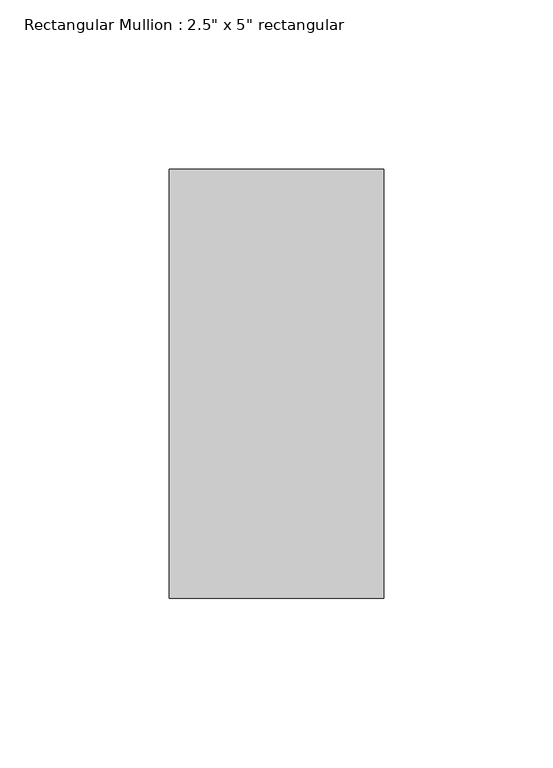
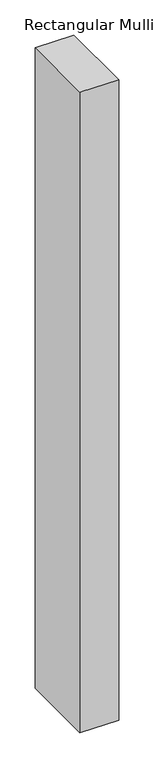
"""IFC4 building model written with IfcOpenShell, lengths in millimetres: member geometry."""

from ifc_helpers import new_model, si_unit, frame, origin, place, context, project, spatial, polyline, outline, extrude, source, transform, mapped, element, save


def member_7ce6cacc(model_context):
    return source(origin(), model_context, "Body", "SweptSolid", [
        extrude(outline(polyline([(31.75, 63.5), (31.75, -63.5), (-31.75, -63.5), (-31.75, 63.5), (31.75, 63.5)])), frame((0.0, 0.0, -1111.25), z_axis=(0.0, 0.0, 1.0), x_axis=(1.0, 0.0, 0.0)), (0.0, 0.0, 1.0), 1111.25),
    ])


if __name__ == "__main__":
    model = new_model("IFC4")
    model_context = context("Model", 3, world=origin())
    ifc_project = project(units=[si_unit("LENGTHUNIT", "METRE", prefix="MILLI")], contexts=[model_context])
    site = spatial("IfcSite", under=ifc_project)
    building = spatial("IfcBuilding", under=site)
    placement = place(None, origin())
    member_shape = member_7ce6cacc(model_context)
    element("IfcMember", 1, ObjectType="Rectangular Mullion : 2.5\" x 5\" rectangular", at=placement, inside=building, context=model_context, shape_type="MappedRepresentation", body=[
        mapped(member_shape, transform((0.0, 0.0, 0.0), x_axis=(1.0, 0.0, 0.0), y_axis=(0.0, 1.0, 0.0), z_axis=(0.0, 0.0, 1.0))),
    ])
    save(model, "model.ifc")

# Revit data of these elements
# Type "Rectangular Mullion : 2.5\" x 5\" rectangular"
#   built-in parameter 1007304 = 0.416667 (stored number, unit not read)
#   built-in parameter 1007301 = 0.104167 (stored number, unit not read)
#   built-in parameter 1007300 = 0.104167 (stored number, unit not read)
# Element 1 (IfcMember, "Rectangular Mullion : 2.5\" x 5\" rectangular")
#   Materials on its faces: "Aluminum"
# Materials
#   "Aluminum": class "Metal", colour RGB 247 247 247, transparency 0, Description = "Aluminum 6061", Cost = 0
